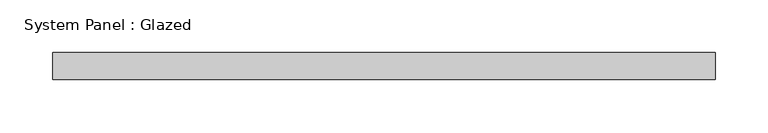
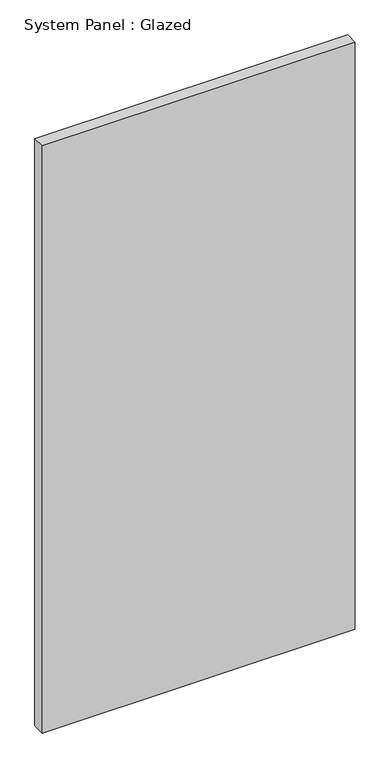
"""IFC4 building model written with IfcOpenShell, lengths in millimetres: plate geometry, System Panel : Glazed."""

from ifc_helpers import new_model, si_unit, origin, origin_with_axes, place, context, project, spatial, polyline, outline, extrude, source, transform, mapped, element, save


def system_panel_glazed_9e0010b7(model_context):
    return source(origin(), model_context, "Body", "SweptSolid", [
        extrude(outline(polyline([(312.335424, 19.05), (-312.335424, 19.05), (-312.335424, 44.45), (312.335424, 44.45), (312.335424, 19.05)])), origin_with_axes(), (0.0, 0.0, 1.0), 1238.4610041),
    ])


if __name__ == "__main__":
    model = new_model("IFC4")
    model_context = context("Model", 3, world=origin())
    ifc_project = project(units=[si_unit("LENGTHUNIT", "METRE", prefix="MILLI")], contexts=[model_context])
    site = spatial("IfcSite", under=ifc_project)
    building = spatial("IfcBuilding", under=site)
    placement = place(None, origin())
    system_panel_glazed_shape = system_panel_glazed_9e0010b7(model_context)
    element("IfcPlate", 1, ObjectType="System Panel : Glazed", at=placement, inside=building, context=model_context, shape_type="MappedRepresentation", body=[
        mapped(system_panel_glazed_shape, transform((0.0, 0.0, 0.0), x_axis=(1.0, 0.0, 0.0), y_axis=(0.0, 1.0, 0.0), z_axis=(0.0, 0.0, 1.0))),
    ])
    save(model, "model.ifc")

# Revit data of these elements
# Type "System Panel : Glazed"
#   Construction Type Id = "GSP4R"
#   Analytic Construction = "1/8 in Pilkington single glazing"
#   Visual Light Transmittance = 0.9
#   Solar Heat Gain Coefficient = 0.86
#   Heat Transfer Coefficient (U) = 1.18115 BTU/(h·ft²·°F)
#   Define Thermal Properties by = 1
# Element 1 (IfcPlate, "System Panel : Glazed")
#   Materials on its faces: "Glass"
# Materials
#   "Glass": class "Glass", colour RGB 0 128 192, transparency 0.75, Description = "Soda Lime Glass", Cost = 0
